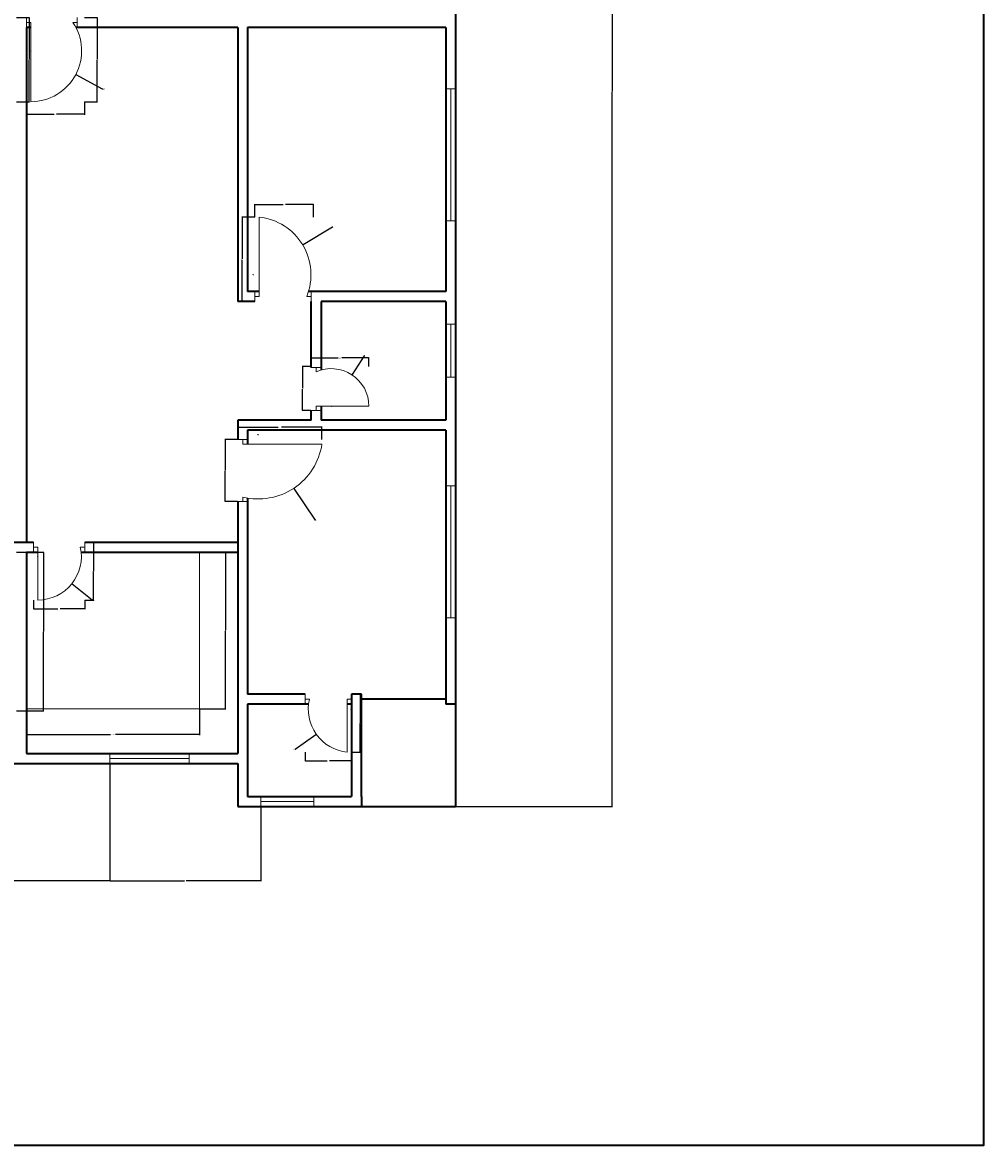
# Model space of a CAD drawing. Units: inches. Extents: x 992 to 2287, y 1476 to 2866.
# Tile 5 of 9: x 1851 to 2287, y 1476 to 1987. Entities that reach past the tile are written whole.
import ezdxf

# ---------------------------------------------------------------- set-up
doc = ezdxf.new("R2010")
doc.units = ezdxf.units.IN
for name, color, linetype, lineweight in [('A-ANNO-DIMS', 2, 'Continuous', 18), ('A-ANNO-TTLB', 7, 'Continuous', 35), ('A-DOOR', 3, 'Continuous', 18), ('A-FLOR-CASE', 9, 'Continuous', 18), ('A-GLAZ', 4, 'Continuous', 18), ('A-WALL', 7, 'Continuous', 35)]:
    doc.layers.add(name, color=color, linetype=linetype, lineweight=lineweight)
doc.styles.get("Standard").update_dxf_attribs({"font": 'arial.ttf'})
doc.dimstyles.get("Standard").update_dxf_attribs({"dimtxt": 0.18, "dimasz": 0.18, "dimexe": 0.18, "dimexo": 0.0625, "dimgap": 0.09, "dimtad": 0, "dimtih": 1, "dimtoh": 1, "dimdec": 4, "dimzin": 0, "dimdsep": 46, "dimtxsty": 'Standard', "dimcen": 0.09, "dimadec": 0, "dimazin": 0, "dimtfac": 1, "dimtdec": 4, "dimtofl": 0, "dimtmove": 0, "dimatfit": 3, "dimfxl": 1, "dimtolj": 1, "dimtzin": 0, "dimarcsym": 0})

# ---------------------------------------------------------------- blocks, each defined once
blk = doc.blocks.new('DOOR-SINGLE-36IN-08')
for p, q in [((0, 33.75), (0, 38.25)), ((0, 36), (2, 36)), ((2, 36), (2, 0)), ((23.12, 36), (21.12, 36)), ((23.12, 38.25), (23.12, 33.75)), ((23.12, 33.75), (23.12, 36))]:
    blk.add_line(p, q)
blk.add_arc((2, 23.08), 23.08, 270, 34.0417)
blk = doc.blocks.new('DOOR-SINGLE-36IN-10')
for p, q in [((2, 2.25), (2, 38.25)), ((0, 4.5), (0, 0)), ((0, 0), (0, 2.25)), ((0, 2.25), (2, 2.25)), ((25.57, 2.25), (23.57, 2.25)), ((25.57, 0), (25.57, 4.5))]:
    blk.add_line(p, q)
blk.add_arc((-0.74, 12.15), 26.25, 337.8522, 84.002)
blk = doc.blocks.new('DOOR-SINGLE-24IN-12')
for p, q in [((0, 19.63), (4.5, 19.63)), ((4.5, 19.63), (2.25, 19.63)), ((2.25, 19.63), (2.25, 17.63)), ((2.25, 0), (2.25, 2)), ((2.25, 2), (26.25, 2)), ((4.5, 0), (0, 0)), ((0, 0), (2.25, 0))]:
    blk.add_line(p, q)
blk.add_arc((9.16, 2), 17.09, 0, 113.8439)
blk = doc.blocks.new('DOOR-SINGLE-24IN-13')
for p, q in [((0, 26.33), (0, 21.83)), ((0, 21.83), (0, 24.08)), ((0, 24.08), (2, 24.08)), ((21.14, 24), (19.14, 24)), ((19.14, 24), (19.14, 0))]:
    blk.add_line(p, q)
blk.add_arc((20.98, 19.45), 19.54, 166.3014, 264.5707)
blk = doc.blocks.new('DOOR-SINGLE-24IN-15')
for p, q in [((0, 26.25), (0, 21.75)), ((23.28, 26.25), (23.28, 21.75)), ((0, 21.75), (0, 24)), ((0, 24), (2, 24)), ((2, 24), (2, 0)), ((23.28, 24), (21.28, 24)), ((23.28, 21.75), (23.28, 24.87)), ((23.28, 24.87), (23.28, 24.87)), ((23.28, 24.87), (23.28, 24))]:
    blk.add_line(p, q)
blk.add_arc((2, 19.75), 19.75, 270, 12.442)
blk = doc.blocks.new('DOOR-SINGLE-36IN-18')
for p, q in [((4.5, 28.09), (0, 28.09)), ((0, 28.09), (2.25, 28.09)), ((2.25, 28.09), (2.25, 26.09)), ((2.25, 26.09), (38.25, 26.09)), ((4.5, 0), (0, 0)), ((0, 0), (2.25, 0)), ((2.25, 0), (2.25, 2))]:
    blk.add_line(p, q)
blk.add_arc((9.28, 30.44), 29.3, 256.1264, 351.459)
blk = doc.blocks.new('WINDOW-24IN-A')
for p, q in [((0, 24), (4.5, 24)), ((4.5, 24), (2.25, 24)), ((2.25, 24), (2.25, 0)), ((2.25, 0), (0, 0)), ((0, 0), (4.5, 0))]:
    blk.add_line(p, q)
blk = doc.blocks.new('WINDOW-60IN-B')
for p, q in [((0, 4.5), (0, 0)), ((0, 0), (0, 2.25)), ((0, 2.25), (60, 2.25)), ((60, 2.25), (60, 4.5)), ((60, 4.5), (60, 0))]:
    blk.add_line(p, q)
blk = doc.blocks.new('WINDOW-36IN')
for p, q in [((0, 4.5), (0, 0)), ((0, 0), (0, 2.25)), ((0, 2.25), (36, 2.25)), ((36, 2.25), (36, 4.5)), ((36, 4.5), (36, 0))]:
    blk.add_line(p, q)
blk = doc.blocks.new('WINDOW-24IN-C')
for p, q in [((0, 24), (4.5, 24)), ((4.5, 24), (2.25, 24)), ((2.25, 24), (2.25, 0)), ((4.5, 0), (0, 0)), ((2.25, 0), (4.5, 0))]:
    blk.add_line(p, q)
blk = doc.blocks.new('COUNTER-L-SOUTHEAST')
for p, q in [((78.66, 0), (78.66, 71.1)), ((0, 0), (78.66, 0))]:
    blk.add_line(p, q)
blk = doc.blocks.new('*D61')
at = {"layer": 'A-ANNO-DIMS', "color": 0, "lineweight": -2, "transparency": 16777216}
for p, q in [((1847.96, 1989.04), (1853.81, 1989.04)), ((1853.63, 1988.86), (1853.63, 1970.1)), ((1853.63, 1950.97), (1853.63, 1969.74)), ((1847.96, 1950.79), (1853.81, 1950.79))]:
    blk.add_line(p, q, dxfattribs=at)
at = {"layer": 'A-ANNO-DIMS', "color": 0, "transparency": 16777216}
for points in [[(1853.6, 1988.86), (1853.66, 1988.86), (1853.63, 1989.04)], [(1853.6, 1950.97), (1853.66, 1950.97), (1853.63, 1950.79)]]:
    blk.add_solid(points, dxfattribs=at)
at = {"layer": 'Defpoints', "color": 0, "transparency": 16777216}
for p in [(1847.89, 1989.04), (1853.63, 1989.04), (1847.89, 1950.79)]:
    blk.add_point(p, dxfattribs=at)
at = {"layer": 'A-ANNO-DIMS', "color": 0, "transparency": 16777216, "insert": (1853.63, 1969.92), "char_height": 0.18, "attachment_point": 5}
blk.add_mtext('\\A1;D07 38 TYP.', dxfattribs=at)
blk = doc.blocks.new('*D63')
at = {"layer": 'A-ANNO-DIMS', "color": 0, "lineweight": -2, "transparency": 16777216}
for p, q in [((1878.84, 1989.04), (1884.7, 1989.04)), ((1884.52, 1988.86), (1884.52, 1970.1)), ((1884.52, 1950.97), (1884.52, 1969.74)), ((1878.84, 1950.79), (1884.7, 1950.79))]:
    blk.add_line(p, q, dxfattribs=at)
at = {"layer": 'A-ANNO-DIMS', "color": 0, "transparency": 16777216}
for points in [[(1884.49, 1988.86), (1884.55, 1988.86), (1884.52, 1989.04)], [(1884.49, 1950.97), (1884.55, 1950.97), (1884.52, 1950.79)]]:
    blk.add_solid(points, dxfattribs=at)
at = {"layer": 'Defpoints', "color": 0, "transparency": 16777216}
for p in [(1878.78, 1989.04), (1884.52, 1989.04), (1878.78, 1950.79)]:
    blk.add_point(p, dxfattribs=at)
at = {"layer": 'A-ANNO-DIMS', "color": 0, "transparency": 16777216, "insert": (1884.52, 1969.92), "char_height": 0.18, "attachment_point": 5}
blk.add_mtext('\\A1;D08 38 TYP.', dxfattribs=at)
blk = doc.blocks.new('*D64')
at = {"layer": 'A-ANNO-DIMS', "color": 0, "lineweight": -2, "transparency": 16777216}
for p, q in [((1852.39, 1950.73), (1852.39, 1944.88)), ((1878.78, 1950.73), (1878.78, 1944.88)), ((1852.57, 1945.06), (1865.06, 1945.06)), ((1878.6, 1945.06), (1866.12, 1945.06))]:
    blk.add_line(p, q, dxfattribs=at)
at = {"layer": 'A-ANNO-DIMS', "color": 0, "transparency": 16777216}
for points in [[(1852.57, 1945.09), (1852.57, 1945.03), (1852.39, 1945.06)], [(1878.6, 1945.09), (1878.6, 1945.03), (1878.78, 1945.06)]]:
    blk.add_solid(points, dxfattribs=at)
at = {"layer": 'Defpoints', "color": 0, "transparency": 16777216}
for p in [(1852.39, 1950.79), (1878.78, 1950.79), (1878.78, 1945.06)]:
    blk.add_point(p, dxfattribs=at)
at = {"layer": 'A-ANNO-DIMS', "color": 0, "transparency": 16777216, "insert": (1865.59, 1945.06), "char_height": 0.18, "attachment_point": 5}
blk.add_mtext('\\A1;26 TYP.', dxfattribs=at)
blk = doc.blocks.new('*D67')
at = {"layer": 'A-ANNO-DIMS', "color": 0, "lineweight": -2, "transparency": 16777216}
for p, q in [((1956.11, 1898.29), (1950.25, 1898.29)), ((1950.43, 1898.11), (1950.43, 1879.35)), ((1950.43, 1860.22), (1950.43, 1878.99)), ((1956.11, 1860.04), (1950.25, 1860.04))]:
    blk.add_line(p, q, dxfattribs=at)
at = {"layer": 'A-ANNO-DIMS', "color": 0, "transparency": 16777216}
for points in [[(1950.4, 1898.11), (1950.46, 1898.11), (1950.43, 1898.29)], [(1950.4, 1860.22), (1950.46, 1860.22), (1950.43, 1860.04)]]:
    blk.add_solid(points, dxfattribs=at)
at = {"layer": 'Defpoints', "color": 0, "transparency": 16777216}
for p in [(1950.43, 1898.29), (1956.17, 1898.29), (1956.17, 1860.04)]:
    blk.add_point(p, dxfattribs=at)
at = {"layer": 'A-ANNO-DIMS', "color": 0, "transparency": 16777216, "insert": (1950.43, 1879.17), "char_height": 0.18, "attachment_point": 5}
blk.add_mtext('\\A1;D10 38 TYP.', dxfattribs=at)
blk = doc.blocks.new('*D68')
at = {"layer": 'A-ANNO-DIMS', "color": 0, "lineweight": -2, "transparency": 16777216}
for p, q in [((1956.17, 1898.36), (1956.17, 1904.21)), ((1956.35, 1904.03), (1968.98, 1904.03)), ((1982.67, 1904.03), (1970.04, 1904.03)), ((1982.85, 1898.36), (1982.85, 1904.21))]:
    blk.add_line(p, q, dxfattribs=at)
at = {"layer": 'A-ANNO-DIMS', "color": 0, "transparency": 16777216}
for points in [[(1956.35, 1904.06), (1956.35, 1904), (1956.17, 1904.03)], [(1982.67, 1904.06), (1982.67, 1904), (1982.85, 1904.03)]]:
    blk.add_solid(points, dxfattribs=at)
at = {"layer": 'Defpoints', "color": 0, "transparency": 16777216}
for p in [(1982.85, 1904.03), (1956.17, 1898.29), (1982.85, 1898.29)]:
    blk.add_point(p, dxfattribs=at)
at = {"layer": 'A-ANNO-DIMS', "color": 0, "transparency": 16777216, "insert": (1969.51, 1904.03), "char_height": 0.18, "attachment_point": 5}
blk.add_mtext('\\A1;27 TYP.', dxfattribs=at)
blk = doc.blocks.new('*D71')
at = {"layer": 'A-ANNO-DIMS', "color": 0, "lineweight": -2, "transparency": 16777216}
for p, q in [((1981.74, 1830.43), (1981.74, 1834.49)), ((1981.92, 1834.31), (1994.08, 1834.31)), ((2007.81, 1834.31), (1995.65, 1834.31)), ((2007.99, 1830.43), (2007.99, 1834.49))]:
    blk.add_line(p, q, dxfattribs=at)
at = {"layer": 'A-ANNO-DIMS', "color": 0, "transparency": 16777216}
for points in [[(1981.92, 1834.34), (1981.92, 1834.28), (1981.74, 1834.31)], [(2007.81, 1834.34), (2007.81, 1834.28), (2007.99, 1834.31)]]:
    blk.add_solid(points, dxfattribs=at)
at = {"layer": 'Defpoints', "color": 0, "transparency": 16777216}
for p in [(2007.99, 1834.31), (1981.74, 1830.37), (2007.99, 1830.37)]:
    blk.add_point(p, dxfattribs=at)
at = {"layer": 'A-ANNO-DIMS', "color": 0, "transparency": 16777216, "insert": (1994.87, 1834.31), "char_height": 0.18, "attachment_point": 5}
blk.add_mtext('\\A1;D12 26 TYP.', dxfattribs=at)
blk = doc.blocks.new('*D72')
at = {"layer": 'A-ANNO-DIMS', "color": 0, "lineweight": -2, "transparency": 16777216}
for p, q in [((1981.68, 1830.37), (1977.62, 1830.37)), ((1977.8, 1830.19), (1977.8, 1820.57)), ((1977.8, 1810.58), (1977.8, 1820.21)), ((1981.68, 1810.4), (1977.62, 1810.4))]:
    blk.add_line(p, q, dxfattribs=at)
at = {"layer": 'A-ANNO-DIMS', "color": 0, "transparency": 16777216}
for points in [[(1977.77, 1830.19), (1977.83, 1830.19), (1977.8, 1830.37)], [(1977.77, 1810.58), (1977.83, 1810.58), (1977.8, 1810.4)]]:
    blk.add_solid(points, dxfattribs=at)
at = {"layer": 'Defpoints', "color": 0, "transparency": 16777216}
for p in [(1977.8, 1830.37), (1981.74, 1830.37), (1981.74, 1810.4)]:
    blk.add_point(p, dxfattribs=at)
at = {"layer": 'A-ANNO-DIMS', "color": 0, "transparency": 16777216, "insert": (1977.8, 1820.39), "char_height": 0.18, "attachment_point": 5}
blk.add_mtext('\\A1;20 TYP.', dxfattribs=at)
blk = doc.blocks.new('*D73')
at = {"layer": 'A-ANNO-DIMS', "color": 0, "lineweight": -2, "transparency": 16777216}
for p, q in [((2000.21, 1681.54), (2004.27, 1681.54)), ((2004.09, 1681.36), (2004.09, 1668.56)), ((2004.09, 1655.39), (2004.09, 1668.2)), ((2000.21, 1655.21), (2004.27, 1655.21))]:
    blk.add_line(p, q, dxfattribs=at)
at = {"layer": 'A-ANNO-DIMS', "color": 0, "transparency": 16777216}
for points in [[(2004.06, 1681.36), (2004.12, 1681.36), (2004.09, 1681.54)], [(2004.06, 1655.39), (2004.12, 1655.39), (2004.09, 1655.21)]]:
    blk.add_solid(points, dxfattribs=at)
at = {"layer": 'Defpoints', "color": 0, "transparency": 16777216}
for p in [(2000.14, 1681.54), (2004.09, 1681.54), (2000.14, 1655.21)]:
    blk.add_point(p, dxfattribs=at)
at = {"layer": 'A-ANNO-DIMS', "color": 0, "transparency": 16777216, "insert": (2004.09, 1668.38), "char_height": 0.18, "attachment_point": 5}
blk.add_mtext('\\A1;D13 26 TYP.', dxfattribs=at)
blk = doc.blocks.new('*D74')
at = {"layer": 'A-ANNO-DIMS', "color": 0, "lineweight": -2, "transparency": 16777216}
for p, q in [((1979.01, 1655.15), (1979.01, 1651.08)), ((2000.14, 1655.15), (2000.14, 1651.08)), ((1979.19, 1651.26), (1989.05, 1651.26)), ((1999.96, 1651.26), (1990.11, 1651.26))]:
    blk.add_line(p, q, dxfattribs=at)
at = {"layer": 'A-ANNO-DIMS', "color": 0, "transparency": 16777216}
for points in [[(1979.19, 1651.29), (1979.19, 1651.23), (1979.01, 1651.26)], [(1999.96, 1651.29), (1999.96, 1651.23), (2000.14, 1651.26)]]:
    blk.add_solid(points, dxfattribs=at)
at = {"layer": 'Defpoints', "color": 0, "transparency": 16777216}
for p in [(1979.01, 1655.21), (2000.14, 1655.21), (2000.14, 1651.26)]:
    blk.add_point(p, dxfattribs=at)
at = {"layer": 'A-ANNO-DIMS', "color": 0, "transparency": 16777216, "insert": (1989.58, 1651.26), "char_height": 0.18, "attachment_point": 5}
blk.add_mtext('\\A1;21 TYP.', dxfattribs=at)
blk = doc.blocks.new('*D77')
at = {"layer": 'A-ANNO-DIMS', "color": 0, "lineweight": -2, "transparency": 16777216}
for p, q in [((1878.94, 1750.54), (1883, 1750.54)), ((1882.82, 1750.36), (1882.82, 1737.6)), ((1882.82, 1724.47), (1882.82, 1737.24)), ((1878.94, 1724.29), (1883, 1724.29))]:
    blk.add_line(p, q, dxfattribs=at)
at = {"layer": 'A-ANNO-DIMS', "color": 0, "transparency": 16777216}
for points in [[(1882.79, 1750.36), (1882.85, 1750.36), (1882.82, 1750.54)], [(1882.79, 1724.47), (1882.85, 1724.47), (1882.82, 1724.29)]]:
    blk.add_solid(points, dxfattribs=at)
at = {"layer": 'Defpoints', "color": 0, "transparency": 16777216}
for p in [(1878.88, 1750.54), (1882.82, 1750.54), (1878.88, 1724.29)]:
    blk.add_point(p, dxfattribs=at)
at = {"layer": 'A-ANNO-DIMS', "color": 0, "transparency": 16777216, "insert": (1882.82, 1737.42), "char_height": 0.18, "attachment_point": 5}
blk.add_mtext('\\A1;D15 26 TYP.', dxfattribs=at)
blk = doc.blocks.new('*D78')
at = {"layer": 'A-ANNO-DIMS', "color": 0, "lineweight": -2, "transparency": 16777216}
for p, q in [((1855.6, 1724.23), (1855.6, 1720.18)), ((1855.78, 1720.36), (1866.71, 1720.36)), ((1878.7, 1720.36), (1867.77, 1720.36)), ((1878.88, 1724.23), (1878.88, 1720.18))]:
    blk.add_line(p, q, dxfattribs=at)
at = {"layer": 'A-ANNO-DIMS', "color": 0, "transparency": 16777216}
for points in [[(1855.78, 1720.39), (1855.78, 1720.33), (1855.6, 1720.36)], [(1878.7, 1720.39), (1878.7, 1720.33), (1878.88, 1720.36)]]:
    blk.add_solid(points, dxfattribs=at)
at = {"layer": 'Defpoints', "color": 0, "transparency": 16777216}
for p in [(1855.6, 1724.29), (1878.88, 1724.29), (1878.88, 1720.36)]:
    blk.add_point(p, dxfattribs=at)
at = {"layer": 'A-ANNO-DIMS', "color": 0, "transparency": 16777216, "insert": (1867.24, 1720.36), "char_height": 0.18, "attachment_point": 5}
blk.add_mtext('\\A1;23 TYP.', dxfattribs=at)
blk = doc.blocks.new('*D83')
at = {"layer": 'A-ANNO-DIMS', "color": 0, "lineweight": -2, "transparency": 16777216}
for p, q in [((1948.39, 1797.26), (1948.39, 1803.11)), ((1948.57, 1802.93), (1966.73, 1802.93)), ((1986.46, 1802.93), (1968.31, 1802.93)), ((1986.64, 1797.26), (1986.64, 1803.11))]:
    blk.add_line(p, q, dxfattribs=at)
at = {"layer": 'A-ANNO-DIMS', "color": 0, "transparency": 16777216}
for points in [[(1948.57, 1802.96), (1948.57, 1802.9), (1948.39, 1802.93)], [(1986.46, 1802.96), (1986.46, 1802.9), (1986.64, 1802.93)]]:
    blk.add_solid(points, dxfattribs=at)
at = {"layer": 'Defpoints', "color": 0, "transparency": 16777216}
for p in [(1986.64, 1802.93), (1948.39, 1797.2), (1986.64, 1797.2)]:
    blk.add_point(p, dxfattribs=at)
at = {"layer": 'A-ANNO-DIMS', "color": 0, "transparency": 16777216, "insert": (1967.52, 1802.93), "char_height": 0.18, "attachment_point": 5}
blk.add_mtext('\\A1;D18 38 TYP.', dxfattribs=at)
blk = doc.blocks.new('*D84')
at = {"layer": 'A-ANNO-DIMS', "color": 0, "lineweight": -2, "transparency": 16777216}
for p, q in [((1948.33, 1797.2), (1942.48, 1797.2)), ((1942.66, 1797.02), (1942.66, 1783.33)), ((1942.66, 1769.28), (1942.66, 1782.97)), ((1948.33, 1769.1), (1942.48, 1769.1))]:
    blk.add_line(p, q, dxfattribs=at)
at = {"layer": 'A-ANNO-DIMS', "color": 0, "transparency": 16777216}
for points in [[(1942.63, 1797.02), (1942.69, 1797.02), (1942.66, 1797.2)], [(1942.63, 1769.28), (1942.69, 1769.28), (1942.66, 1769.1)]]:
    blk.add_solid(points, dxfattribs=at)
at = {"layer": 'Defpoints', "color": 0, "transparency": 16777216}
for p in [(1942.66, 1797.2), (1948.39, 1797.2), (1948.39, 1769.1)]:
    blk.add_point(p, dxfattribs=at)
at = {"layer": 'A-ANNO-DIMS', "color": 0, "transparency": 16777216, "insert": (1942.66, 1783.15), "char_height": 0.18, "attachment_point": 5}
blk.add_mtext('\\A1;28 TYP.', dxfattribs=at)
blk = doc.blocks.new('*D88')
at = {"layer": 'A-ANNO-DIMS', "color": 0, "lineweight": -2, "transparency": 16777216}
for p, q in [((1847.96, 1746.04), (1860.34, 1746.04)), ((1860.16, 1745.86), (1860.16, 1710.19)), ((1860.16, 1674.16), (1860.16, 1709.83)), ((1847.96, 1673.98), (1860.34, 1673.98))]:
    blk.add_line(p, q, dxfattribs=at)
at = {"layer": 'A-ANNO-DIMS', "color": 0, "transparency": 16777216}
for points in [[(1860.13, 1745.86), (1860.19, 1745.86), (1860.16, 1746.04)], [(1860.13, 1674.16), (1860.19, 1674.16), (1860.16, 1673.98)]]:
    blk.add_solid(points, dxfattribs=at)
at = {"layer": 'Defpoints', "color": 0, "transparency": 16777216}
for p in [(1847.89, 1746.04), (1860.16, 1746.04), (1847.89, 1673.98)]:
    blk.add_point(p, dxfattribs=at)
at = {"layer": 'A-ANNO-DIMS', "color": 0, "transparency": 16777216, "insert": (1860.16, 1710.01), "char_height": 0.18, "attachment_point": 5}
blk.add_mtext('\\A1;72 TYP.', dxfattribs=at)
blk = doc.blocks.new('*D89')
at = {"layer": 'A-ANNO-DIMS', "color": 0, "lineweight": -2, "transparency": 16777216}
for p, q in [((1852.39, 1674.88), (1852.39, 1662.96)), ((1931.05, 1674.88), (1931.05, 1662.96)), ((1852.57, 1663.14), (1890.54, 1663.14)), ((1930.87, 1663.14), (1892.91, 1663.14))]:
    blk.add_line(p, q, dxfattribs=at)
at = {"layer": 'A-ANNO-DIMS', "color": 0, "transparency": 16777216}
for points in [[(1852.57, 1663.17), (1852.57, 1663.11), (1852.39, 1663.14)], [(1930.87, 1663.17), (1930.87, 1663.11), (1931.05, 1663.14)]]:
    blk.add_solid(points, dxfattribs=at)
at = {"layer": 'Defpoints', "color": 0, "transparency": 16777216}
for p in [(1852.39, 1674.94), (1931.05, 1674.94), (1931.05, 1663.14)]:
    blk.add_point(p, dxfattribs=at)
at = {"layer": 'A-ANNO-DIMS', "color": 0, "transparency": 16777216, "insert": (1891.72, 1663.14), "char_height": 0.18, "attachment_point": 5}
blk.add_mtext('\\A1;COUNTER 79 TYP.', dxfattribs=at)
blk = doc.blocks.new('*D90')
at = {"layer": 'A-ANNO-DIMS', "color": 0, "lineweight": -2, "transparency": 16777216}
for p, q in [((1931.11, 1746.04), (1943.03, 1746.04)), ((1942.85, 1745.86), (1942.85, 1710.67)), ((1942.85, 1675.12), (1942.85, 1710.31)), ((1931.11, 1674.94), (1943.03, 1674.94))]:
    blk.add_line(p, q, dxfattribs=at)
at = {"layer": 'A-ANNO-DIMS', "color": 0, "transparency": 16777216}
for points in [[(1942.82, 1745.86), (1942.88, 1745.86), (1942.85, 1746.04)], [(1942.82, 1675.12), (1942.88, 1675.12), (1942.85, 1674.94)]]:
    blk.add_solid(points, dxfattribs=at)
at = {"layer": 'Defpoints', "color": 0, "transparency": 16777216}
for p in [(1931.05, 1746.04), (1942.85, 1746.04), (1931.05, 1674.94)]:
    blk.add_point(p, dxfattribs=at)
at = {"layer": 'A-ANNO-DIMS', "color": 0, "transparency": 16777216, "insert": (1942.85, 1710.49), "char_height": 0.18, "attachment_point": 5}
blk.add_mtext('\\A1;71 TYP.', dxfattribs=at)
blk = doc.blocks.new('*D112')
at = {"layer": 'A-ANNO-DIMS', "color": 0, "lineweight": -2, "transparency": 16777216}
for p, q in [((2047.46, 2280.04), (2118.61, 2280.04)), ((2118.43, 2279.86), (2118.43, 1955.47)), ((2118.43, 1630.72), (2118.43, 1955.11)), ((2047.46, 1630.54), (2118.61, 1630.54))]:
    blk.add_line(p, q, dxfattribs=at)
at = {"layer": 'A-ANNO-DIMS', "color": 0, "transparency": 16777216}
for points in [[(2118.4, 2279.86), (2118.46, 2279.86), (2118.43, 2280.04)], [(2118.4, 1630.72), (2118.46, 1630.72), (2118.43, 1630.54)]]:
    blk.add_solid(points, dxfattribs=at)
at = {"layer": 'Defpoints', "color": 0, "transparency": 16777216}
for p in [(2047.39, 2280.04), (2118.43, 2280.04), (2047.39, 1630.54)]:
    blk.add_point(p, dxfattribs=at)
at = {"layer": 'A-ANNO-DIMS', "color": 0, "transparency": 16777216, "insert": (2118.43, 1955.29), "char_height": 0.18, "attachment_point": 5}
blk.add_mtext('\\A1;649.5', dxfattribs=at)
blk = doc.blocks.new('*D119')
at = {"layer": 'A-ANNO-DIMS', "color": 0, "lineweight": -2, "transparency": 16777216}
for p, q in [((1775.9, 1649.98), (1775.9, 1596.56)), ((1890.29, 1649.98), (1890.29, 1596.56)), ((1776.08, 1596.74), (1832.71, 1596.74)), ((1890.11, 1596.74), (1833.48, 1596.74))]:
    blk.add_line(p, q, dxfattribs=at)
at = {"layer": 'A-ANNO-DIMS', "color": 0, "transparency": 16777216}
for points in [[(1776.08, 1596.77), (1776.08, 1596.71), (1775.9, 1596.74)], [(1890.11, 1596.77), (1890.11, 1596.71), (1890.29, 1596.74)]]:
    blk.add_solid(points, dxfattribs=at)
at = {"layer": 'Defpoints', "color": 0, "transparency": 16777216}
for p in [(1775.9, 1650.04), (1890.29, 1650.04), (1890.29, 1596.74)]:
    blk.add_point(p, dxfattribs=at)
at = {"layer": 'A-ANNO-DIMS', "color": 0, "transparency": 16777216, "insert": (1833.1, 1596.74), "char_height": 0.18, "attachment_point": 5}
blk.add_mtext('\\A1;114.4', dxfattribs=at)
blk = doc.blocks.new('*D120')
at = {"layer": 'A-ANNO-DIMS', "color": 0, "lineweight": -2, "transparency": 16777216}
for p, q in [((1890.29, 1649.98), (1890.29, 1596.56)), ((1958.96, 1630.48), (1958.96, 1596.56)), ((1890.47, 1596.74), (1924.23, 1596.74)), ((1958.78, 1596.74), (1925.02, 1596.74))]:
    blk.add_line(p, q, dxfattribs=at)
at = {"layer": 'A-ANNO-DIMS', "color": 0, "transparency": 16777216}
for points in [[(1890.47, 1596.77), (1890.47, 1596.71), (1890.29, 1596.74)], [(1958.78, 1596.77), (1958.78, 1596.71), (1958.96, 1596.74)]]:
    blk.add_solid(points, dxfattribs=at)
at = {"layer": 'Defpoints', "color": 0, "transparency": 16777216}
for p in [(1890.29, 1650.04), (1958.96, 1630.54), (1958.96, 1596.74)]:
    blk.add_point(p, dxfattribs=at)
at = {"layer": 'A-ANNO-DIMS', "color": 0, "transparency": 16777216, "insert": (1924.63, 1596.74), "char_height": 0.18, "attachment_point": 5}
blk.add_mtext('\\A1;68.67', dxfattribs=at)
blk = doc.blocks.new('*D155')
at = {"layer": 'A-ANNO-DIMS', "color": 0, "lineweight": -2, "transparency": 16777216}
for p, q in [((1957.58, 1799.55), (1957.76, 1799.55)), ((1957.67, 1799.46), (1957.67, 1799.64)), ((1983.74, 1760.59), (1974.07, 1775.05)), ((1983.92, 1760.59), (1983.74, 1760.59))]:
    blk.add_line(p, q, dxfattribs=at)
at = {"layer": 'A-ANNO-DIMS', "color": 0, "transparency": 16777216}
blk.add_solid([(1974.09, 1775.07), (1974.04, 1775.03), (1973.97, 1775.2)], dxfattribs=at)
at = {"layer": 'Defpoints', "color": 0, "transparency": 16777216}
for p in [(1957.67, 1799.55), (1973.97, 1775.2)]:
    blk.add_point(p, dxfattribs=at)
at = {"layer": 'A-ANNO-DIMS', "color": 0, "transparency": 16777216, "insert": (1984.33, 1760.59), "char_height": 0.18, "attachment_point": 5}
blk.add_mtext('\\A1;R29.3', dxfattribs=at)
blk = doc.blocks.new('*D157')
at = {"layer": 'A-ANNO-DIMS', "color": 0, "lineweight": -2, "transparency": 16777216}
for p, q in [((1991.46, 1893.77), (1978.1, 1885.77)), ((1991.64, 1893.77), (1991.46, 1893.77)), ((1955.34, 1872.19), (1955.52, 1872.19)), ((1955.43, 1872.1), (1955.43, 1872.28))]:
    blk.add_line(p, q, dxfattribs=at)
at = {"layer": 'A-ANNO-DIMS', "color": 0, "transparency": 16777216}
blk.add_solid([(1978.08, 1885.8), (1978.12, 1885.75), (1977.95, 1885.68)], dxfattribs=at)
at = {"layer": 'Defpoints', "color": 0, "transparency": 16777216}
for p in [(1977.95, 1885.68), (1955.43, 1872.19)]:
    blk.add_point(p, dxfattribs=at)
at = {"layer": 'A-ANNO-DIMS', "color": 0, "transparency": 16777216, "insert": (1992.12, 1893.77), "char_height": 0.18, "attachment_point": 5}
blk.add_mtext('\\A1;R26.25', dxfattribs=at)
blk = doc.blocks.new('*D159')
at = {"layer": 'A-ANNO-DIMS', "color": 0, "lineweight": -2, "transparency": 16777216}
for p, q in [((1854.3, 1973.87), (1854.48, 1973.87)), ((1854.39, 1973.78), (1854.39, 1973.96)), ((1887.01, 1956.55), (1874.94, 1962.96)), ((1887.19, 1956.55), (1887.01, 1956.55))]:
    blk.add_line(p, q, dxfattribs=at)
at = {"layer": 'A-ANNO-DIMS', "color": 0, "transparency": 16777216}
blk.add_solid([(1874.95, 1962.99), (1874.92, 1962.93), (1874.78, 1963.04)], dxfattribs=at)
at = {"layer": 'Defpoints', "color": 0, "transparency": 16777216}
for p in [(1854.39, 1973.87), (1874.78, 1963.04)]:
    blk.add_point(p, dxfattribs=at)
at = {"layer": 'A-ANNO-DIMS', "color": 0, "transparency": 16777216, "insert": (1887.67, 1956.55), "char_height": 0.18, "attachment_point": 5}
blk.add_mtext('\\A1;R23.08', dxfattribs=at)
blk = doc.blocks.new('*D162')
at = {"layer": 'A-ANNO-DIMS', "color": 0, "lineweight": -2, "transparency": 16777216}
for p, q in [((1857.51, 1744.04), (1857.69, 1744.04)), ((1857.6, 1743.95), (1857.6, 1744.13)), ((1882.23, 1724.25), (1873.13, 1731.56)), ((1882.41, 1724.25), (1882.23, 1724.25))]:
    blk.add_line(p, q, dxfattribs=at)
at = {"layer": 'A-ANNO-DIMS', "color": 0, "transparency": 16777216}
blk.add_solid([(1873.15, 1731.58), (1873.11, 1731.53), (1872.99, 1731.67)], dxfattribs=at)
at = {"layer": 'Defpoints', "color": 0, "transparency": 16777216}
for p in [(1857.6, 1744.04), (1872.99, 1731.67)]:
    blk.add_point(p, dxfattribs=at)
at = {"layer": 'A-ANNO-DIMS', "color": 0, "transparency": 16777216, "insert": (1882.96, 1724.25), "char_height": 0.18, "attachment_point": 5}
blk.add_mtext('\\A1;R19.746', dxfattribs=at)
blk = doc.blocks.new('*D163')
at = {"layer": 'A-ANNO-DIMS', "color": 0, "lineweight": -2, "transparency": 16777216}
for p, q in [((1999.9, 1674.67), (2000.08, 1674.67)), ((1999.99, 1674.58), (1999.99, 1674.76)), ((1974.52, 1656.54), (1983.93, 1663.23)), ((1974.34, 1656.54), (1974.52, 1656.54))]:
    blk.add_line(p, q, dxfattribs=at)
at = {"layer": 'A-ANNO-DIMS', "color": 0, "transparency": 16777216}
blk.add_solid([(1983.91, 1663.26), (1983.94, 1663.21), (1984.07, 1663.34)], dxfattribs=at)
at = {"layer": 'Defpoints', "color": 0, "transparency": 16777216}
for p in [(1999.99, 1674.67), (1984.07, 1663.34)]:
    blk.add_point(p, dxfattribs=at)
at = {"layer": 'A-ANNO-DIMS', "color": 0, "transparency": 16777216, "insert": (1973.86, 1656.54), "char_height": 0.18, "attachment_point": 5}
blk.add_mtext('\\A1;R19.54', dxfattribs=at)
blk = doc.blocks.new('*D168')
at = {"layer": 'A-ANNO-DIMS', "color": 0, "lineweight": -2, "transparency": 16777216}
for p, q in [((2005.82, 1835.32), (2000.33, 1826.87)), ((2006, 1835.32), (2005.82, 1835.32)), ((1990.81, 1812.4), (1990.99, 1812.4)), ((1990.9, 1812.31), (1990.9, 1812.49))]:
    blk.add_line(p, q, dxfattribs=at)
at = {"layer": 'A-ANNO-DIMS', "color": 0, "transparency": 16777216}
blk.add_solid([(2000.3, 1826.89), (2000.35, 1826.86), (2000.23, 1826.72)], dxfattribs=at)
at = {"layer": 'Defpoints', "color": 0, "transparency": 16777216}
for p in [(2000.23, 1826.72), (1990.9, 1812.4)]:
    blk.add_point(p, dxfattribs=at)
at = {"layer": 'A-ANNO-DIMS', "color": 0, "transparency": 16777216, "insert": (2006.48, 1835.32), "char_height": 0.18, "attachment_point": 5}
blk.add_mtext('\\A1;R17.09', dxfattribs=at)

msp = doc.modelspace()

# ---------------------------------------------------------------- linework, layer by layer
at = {"layer": 'A-ANNO-TTLB'}
msp.add_lwpolyline([(992.3484, 2866.1952), (2287.217, 2866.1952), (2287.217, 1476.4066), (992.3484, 1476.4066)], close=True, dxfattribs=at)
at = {"layer": 'A-WALL'}
for p, q in [((2047.3946, 2280.0428), (2047.3946, 1677.0428)), ((2047.3946, 1989.0428), (2047.3946, 1984.5428)), ((1852.3946, 1984.5428), (1852.3946, 1750.5428)), ((1854.3946, 1984.5428), (1852.3946, 1984.5428)), ((1948.3946, 1984.5428), (1874.86, 1984.5428)), ((1948.3946, 1984.5428), (1948.3946, 1860.0428)), ((1952.8946, 1984.5428), (1952.8946, 1864.5428)), ((2042.8946, 1984.5428), (1952.8946, 1984.5428)), ((2042.8946, 1984.5428), (2042.8946, 1864.5428)), ((1958.1719, 1864.5428), (1952.8946, 1864.5428)), ((2042.8946, 1864.5428), (1980.5392, 1864.5428)), ((1956.1719, 1860.0428), (1948.3946, 1860.0428)), ((1981.7406, 1830.0352), (1981.7406, 1860.0428)), ((2042.8946, 1860.0428), (1986.2406, 1860.0428)), ((2042.8946, 1860.0428), (1986.2406, 1860.0428)), ((1986.2406, 1860.0428), (1986.2406, 1828.8466)), ((2042.8946, 1860.0428), (2042.8946, 1806.0428)), ((1986.2406, 1812.4029), (1986.2406, 1806.0428)), ((1981.7406, 1806.0428), (1981.7406, 1810.4029)), ((1948.3946, 1806.0428), (1948.3946, 1797.1964)), ((1981.7406, 1806.0428), (1948.3946, 1806.0428)), ((2042.8946, 1806.0428), (1986.2406, 1806.0428)), ((1952.8946, 1801.5428), (1952.8946, 1795.1964)), ((2042.8946, 1801.5428), (1952.8946, 1801.5428)), ((2042.8946, 1801.5428), (2042.8946, 1681.5428)), ((1948.3946, 1769.1032), (1948.3946, 1654.5428)), ((1952.8946, 1770.6402), (1952.8946, 1681.5428)), ((1844.22, 1750.5428), (1855.598, 1750.5428)), ((1852.3946, 1746.0428), (1857.598, 1746.0428)), ((1852.3946, 1746.0428), (1852.3946, 1654.5428)), ((1877.2418, 1746.0428), (1948.3946, 1746.0428)), ((1878.88, 1750.5428), (1948.3946, 1750.5428)), ((1979.0092, 1681.5428), (1952.8946, 1681.5428)), ((2004.6446, 1681.5428), (2000.1446, 1681.5428)), ((2000.1446, 1681.5428), (2000.1446, 1635.0428)), ((2004.6446, 1635.0428), (2004.6446, 1681.5428)), ((2042.8946, 1679.2928), (2004.6446, 1679.2928)), ((2042.8946, 1681.5428), (2042.8946, 1677.0428)), ((1952.8946, 1677.0428), (1952.8946, 1635.0428)), ((1980.5985, 1677.0428), (1952.8946, 1677.0428)), ((2000.1446, 1677.0428), (1998.1446, 1677.0428)), ((2000.1446, 1677.0428), (1998.1446, 1677.0428)), ((2047.3946, 1677.0428), (2042.8946, 1677.0428)), ((2047.3946, 1677.0428), (2047.3946, 1631.5386)), ((1852.3946, 1654.5428), (1948.3946, 1654.5428)), ((1748.1835, 1650.0428), (1948.3946, 1650.0428)), ((1948.3946, 1650.0428), (1948.3946, 1630.5428)), ((1952.8946, 1635.0428), (2000.1446, 1635.0428)), ((2004.6446, 1635.0428), (2004.6446, 1630.5428)), ((1948.3946, 1630.5428), (2047.3946, 1630.5428)), ((2047.3946, 1631.5386), (2047.3946, 1630.5428))]:
    msp.add_line(p, q, dxfattribs=at)

# ---------------------------------------------------------------- block references
at = {"layer": 'A-DOOR'}
for name, p in [('DOOR-SINGLE-36IN-08', (1852.395, 1950.793)), ('DOOR-SINGLE-36IN-10', (1956.172, 1860.043)), ('DOOR-SINGLE-24IN-12', (1981.741, 1810.403)), ('DOOR-SINGLE-36IN-18', (1948.395, 1769.103)), ('DOOR-SINGLE-24IN-15', (1855.598, 1724.293)), ('DOOR-SINGLE-24IN-13', (1979.009, 1655.213))]:
    msp.add_blockref(name, p, dxfattribs=at)
at = {"layer": 'A-FLOR-CASE'}
msp.add_blockref('COUNTER-L-SOUTHEAST', (1852.395, 1674.941), dxfattribs=at)
at = {"layer": 'A-GLAZ', "rotation": 90}
for p in [(2047.3944, 1896.7008), (2047.3944, 1716.1491)]:
    msp.add_blockref('WINDOW-60IN-B', p, dxfattribs=at)
at = {"layer": 'A-GLAZ'}
msp.add_blockref('WINDOW-24IN-C', (2042.895, 1825.649), dxfattribs=at)
at = {"layer": 'A-GLAZ', "extrusion": (0, 0, -1), "zscale": -1}
for name, p, rotation in [('WINDOW-36IN', (-1890.2945, 1654.5426), 180), ('WINDOW-24IN-A', (-1958.9605, 1630.5432), 90)]:
    msp.add_blockref(name, p, dxfattribs=dict(at, rotation=rotation))

# ---------------------------------------------------------------- dimensions: what is measured, and where the dimension line sits
at = {"layer": 'A-ANNO-DIMS'}
dim = msp.add_linear_dim(base=(2118.4292, 2280.0428), p1=(2047.3946, 1630.5428), p2=(2047.3946, 2280.0428), angle=90, dimstyle='Standard', override={"dimdec": 1, "dimlfac": 1, "dimrnd": 0, "dimzin": 0, "dimdsep": 46, "dimlunit": 2}, dxfattribs=at)
dim.commit()
dim.dimension.update_dxf_attribs({"geometry": '*D112', "text_midpoint": (2118.4292, 1955.2928)})
for base, p1, p2, text, picture, middle in [((1853.6321, 1989.0428), (1847.8946, 1950.7928), (1847.8946, 1989.0428), 'D07 <> TYP.', '*D61', (1853.6321, 1969.9178)), ((1884.5196, 1989.0428), (1878.7821, 1950.7928), (1878.7821, 1989.0428), 'D08 <> TYP.', '*D63', (1884.5196, 1969.9178)), ((1950.4344, 1898.2928), (1956.1719, 1860.0428), (1956.1719, 1898.2928), 'D10 <> TYP.', '*D67', (1950.4344, 1879.1678)), ((1977.8031, 1830.3714), (1981.7406, 1810.4029), (1981.7406, 1830.3714), '<> TYP.', '*D72', (1977.8031, 1820.3871)), ((1942.6571, 1797.1964), (1948.3946, 1769.1032), (1948.3946, 1797.1964), '<> TYP.', '*D84', (1942.6571, 1783.1498)), ((1860.1607, 1746.0428), (1847.8946, 1673.9844), (1847.8946, 1746.0428), '<> TYP.', '*D88', (1860.1607, 1710.0136)), ((1882.8175, 1750.5428), (1878.88, 1724.2928), (1878.88, 1750.5428), 'D15 <> TYP.', '*D77', (1882.8175, 1737.4178)), ((1942.8501, 1746.0428), (1931.0515, 1674.9413), (1931.0515, 1746.0428), '<> TYP.', '*D90', (1942.8501, 1710.492)), ((2004.0941, 1681.5428), (2000.1446, 1655.213), (2000.1446, 1681.5428), 'D13 <> TYP.', '*D73', (2004.0941, 1668.3779))]:
    dim = msp.add_linear_dim(base=base, p1=p1, p2=p2, angle=90, text=text, dimstyle='Standard', override={"dimdec": 0, "dimlfac": 1, "dimrnd": 0, "dimzin": 0, "dimdsep": 46, "dimlunit": 2}, dxfattribs=at)
    dim.commit()
    dim.dimension.update_dxf_attribs({"geometry": picture, "text_midpoint": middle})
for center, mpoint, override, picture, middle in [((1854.3946, 1973.8727), (1874.777, 1963.045), {"dimdec": 2, "dimlfac": 1, "dimrnd": 0, "dimzin": 0, "dimdsep": 46, "dimlunit": 2}, '*D159', (1887.6665, 1956.5483)), ((1955.4291, 1872.1883), (1977.9455, 1885.6783), {"dimdec": 2, "dimlfac": 1, "dimrnd": 0, "dimzin": 0, "dimdsep": 46, "dimlunit": 2}, '*D157', (1992.1158, 1893.7723)), ((1990.8996, 1812.4029), (2000.2278, 1826.7237), {"dimdec": 2, "dimlfac": 1, "dimrnd": 0, "dimzin": 0, "dimdsep": 46, "dimlunit": 2}, '*D168', (2006.4848, 1835.3162)), ((1957.6701, 1799.5479), (1973.9659, 1775.1982), {"dimdec": 1, "dimlfac": 1, "dimrnd": 0, "dimzin": 0, "dimdsep": 46, "dimlunit": 2}, '*D155', (1984.3332, 1760.5884)), ((1857.598, 1744.0385), (1872.9909, 1731.6711), {"dimdec": 3, "dimlfac": 1, "dimrnd": 0, "dimzin": 0, "dimdsep": 46, "dimlunit": 2}, '*D162', (1882.9563, 1724.2506)), ((1999.9934, 1674.6654), (1984.073, 1663.336), {"dimdec": 2, "dimlfac": 1, "dimrnd": 0, "dimzin": 0, "dimdsep": 46, "dimlunit": 2}, '*D163', (1973.8613, 1656.5384))]:
    dim = msp.add_radius_dim(center=center, mpoint=mpoint, dimstyle='Standard', override=override, dxfattribs=at)
    dim.commit()
    dim.dimension.update_dxf_attribs({"geometry": picture, "text_midpoint": middle, "dimtype": 164})
for base, p1, p2, text, picture, middle in [((1878.7821, 1945.0553), (1852.3946, 1950.7928), (1878.7821, 1950.7928), '<> TYP.', '*D64', (1865.5884, 1945.0553)), ((1982.8519, 1904.0303), (1956.1719, 1898.2928), (1982.8519, 1898.2928), '<> TYP.', '*D68', (1969.5119, 1904.0303)), ((2007.9906, 1834.3089), (1981.7406, 1830.3714), (2007.9906, 1830.3714), 'D12 <> TYP.', '*D71', (1994.8656, 1834.3089)), ((1986.6446, 1802.9339), (1948.3946, 1797.1964), (1986.6446, 1797.1964), 'D18 <> TYP.', '*D83', (1967.5196, 1802.9339)), ((1878.88, 1720.3553), (1855.598, 1724.2928), (1878.88, 1724.2928), '<> TYP.', '*D78', (1867.239, 1720.3553)), ((1931.0515, 1663.1427), (1852.3946, 1674.9413), (1931.0515, 1674.9413), 'COUNTER <> TYP.', '*D89', (1891.7231, 1663.1427)), ((2000.1446, 1651.2636), (1979.0092, 1655.213), (2000.1446, 1655.213), '<> TYP.', '*D74', (1989.5769, 1651.2636))]:
    dim = msp.add_linear_dim(base=base, p1=p1, p2=p2, text=text, dimstyle='Standard', override={"dimdec": 0, "dimlfac": 1, "dimrnd": 0, "dimzin": 0, "dimdsep": 46, "dimlunit": 2}, dxfattribs=at)
    dim.commit()
    dim.dimension.update_dxf_attribs({"geometry": picture, "text_midpoint": middle})
for base, p1, p2, override, picture, middle in [((1890.2943, 1596.7428), (1775.9038, 1650.0428), (1890.2943, 1650.0428), {"dimdec": 1, "dimlfac": 1, "dimrnd": 0, "dimzin": 0, "dimdsep": 46, "dimlunit": 2}, '*D119', (1833.0991, 1596.7428)), ((1958.9602, 1596.7428), (1890.2943, 1650.0428), (1958.9602, 1630.5428), {"dimdec": 2, "dimlfac": 1, "dimrnd": 0, "dimzin": 0, "dimdsep": 46, "dimlunit": 2}, '*D120', (1924.6273, 1596.7428))]:
    dim = msp.add_linear_dim(base=base, p1=p1, p2=p2, dimstyle='Standard', override=override, dxfattribs=at)
    dim.commit()
    dim.dimension.update_dxf_attribs({"geometry": picture, "text_midpoint": middle})

doc.saveas('drawing.dxf')
